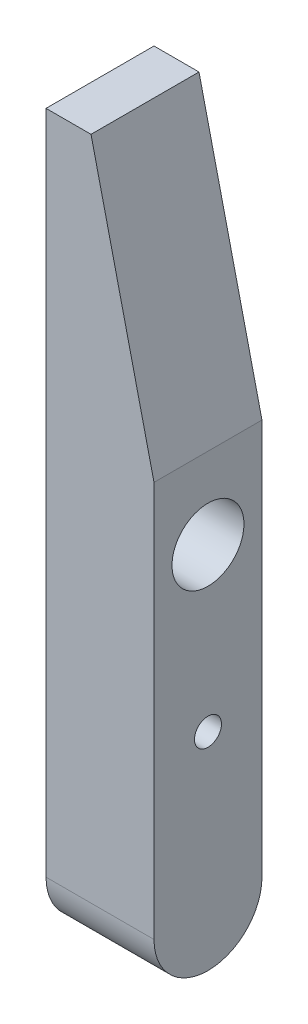
ISO-10303-21;
HEADER;
FILE_DESCRIPTION(('STEP AP214'),'2;1');
FILE_NAME('part.step','',(''),(''),'','','');
FILE_SCHEMA(('AUTOMOTIVE_DESIGN { 1 0 10303 214 1 1 1 1 }'));
ENDSEC;
DATA;
#1=APPLICATION_CONTEXT('core data for automotive mechanical design processes');
#2=APPLICATION_PROTOCOL_DEFINITION('international standard','automotive_design',2000,#1);
#3=PRODUCT_CONTEXT('',#1,'mechanical');
#4=PRODUCT('Part','Part','',(#3));
#5=PRODUCT_RELATED_PRODUCT_CATEGORY('part','',(#4));
#6=PRODUCT_DEFINITION_FORMATION('','',#4);
#7=PRODUCT_DEFINITION_CONTEXT('part definition',#1,'design');
#8=PRODUCT_DEFINITION('design','',#6,#7);
#9=PRODUCT_DEFINITION_SHAPE('','',#8);
#10=(LENGTH_UNIT() NAMED_UNIT(*) SI_UNIT(.MILLI.,.METRE.));
#11=(NAMED_UNIT(*) PLANE_ANGLE_UNIT() SI_UNIT($,.RADIAN.));
#12=(NAMED_UNIT(*) SI_UNIT($,.STERADIAN.) SOLID_ANGLE_UNIT());
#13=UNCERTAINTY_MEASURE_WITH_UNIT(LENGTH_MEASURE(1.E-05),#10,'distance_accuracy_value','');
#14=(GEOMETRIC_REPRESENTATION_CONTEXT(3) GLOBAL_UNCERTAINTY_ASSIGNED_CONTEXT((#13)) GLOBAL_UNIT_ASSIGNED_CONTEXT((#10,
#11,#12)) REPRESENTATION_CONTEXT('',''));
#15=CARTESIAN_POINT('',(0.,0.,0.));
#16=DIRECTION('',(0.,0.,1.));
#17=DIRECTION('',(1.,0.,0.));
#18=AXIS2_PLACEMENT_3D('',#15,#16,#17);
#19=CARTESIAN_POINT('',(0.,-74.,6.));
#20=DIRECTION('',(1.,0.,0.));
#21=DIRECTION('',(0.,0.,-1.));
#22=AXIS2_PLACEMENT_3D('',#19,#20,#21);
#23=PLANE('',#22);
#24=CARTESIAN_POINT('',(0.,-39.,0.));
#25=DIRECTION('',(1.,0.,0.));
#26=DIRECTION('',(0.,0.,-1.));
#27=AXIS2_PLACEMENT_3D('',#24,#25,#26);
#28=CIRCLE('',#27,4.);
#29=CARTESIAN_POINT('',(0.,-39.,-4.));
#30=VERTEX_POINT('',#29);
#31=EDGE_CURVE('E141',#30,#30,#28,.T.);
#32=ORIENTED_EDGE('',*,*,#31,.T.);
#33=EDGE_LOOP('',(#32));
#34=FACE_BOUND('',#33,.T.);
#35=CARTESIAN_POINT('',(0.,-74.,0.));
#36=DIRECTION('',(-1.,0.,0.));
#37=DIRECTION('',(0.,0.,1.));
#38=AXIS2_PLACEMENT_3D('',#35,#36,#37);
#39=CIRCLE('',#38,2.4);
#40=CARTESIAN_POINT('',(0.,-74.,2.4));
#41=VERTEX_POINT('',#40);
#42=EDGE_CURVE('E138',#41,#41,#39,.T.);
#43=ORIENTED_EDGE('',*,*,#42,.F.);
#44=EDGE_LOOP('',(#43));
#45=FACE_BOUND('',#44,.T.);
#46=DIRECTION('',(0.,-1.,0.));
#47=VECTOR('',#46,1.);
#48=CARTESIAN_POINT('',(0.,-74.,-6.));
#49=LINE('',#48,#47);
#50=CARTESIAN_POINT('',(0.,0.,-6.));
#51=VERTEX_POINT('',#50);
#52=CARTESIAN_POINT('',(0.,-74.,-6.));
#53=VERTEX_POINT('',#52);
#54=EDGE_CURVE('E112',#51,#53,#49,.T.);
#55=ORIENTED_EDGE('',*,*,#54,.T.);
#56=CARTESIAN_POINT('',(0.,-74.,0.));
#57=DIRECTION('',(-1.,0.,0.));
#58=DIRECTION('',(0.,0.,1.));
#59=AXIS2_PLACEMENT_3D('',#56,#57,#58);
#60=CIRCLE('',#59,6.);
#61=CARTESIAN_POINT('',(0.,-74.,6.));
#62=VERTEX_POINT('',#61);
#63=EDGE_CURVE('E132',#53,#62,#60,.T.);
#64=ORIENTED_EDGE('',*,*,#63,.T.);
#65=DIRECTION('',(0.,-1.,0.));
#66=VECTOR('',#65,1.);
#67=CARTESIAN_POINT('',(0.,-74.,6.));
#68=LINE('',#67,#66);
#69=CARTESIAN_POINT('',(0.,0.,6.));
#70=VERTEX_POINT('',#69);
#71=EDGE_CURVE('E89',#70,#62,#68,.T.);
#72=ORIENTED_EDGE('',*,*,#71,.F.);
#73=DIRECTION('',(0.,0.,-1.));
#74=VECTOR('',#73,1.);
#75=CARTESIAN_POINT('',(0.,0.,6.));
#76=LINE('',#75,#74);
#77=EDGE_CURVE('E109',#70,#51,#76,.T.);
#78=ORIENTED_EDGE('',*,*,#77,.T.);
#79=EDGE_LOOP('',(#55,#64,#72,#78));
#80=FACE_BOUND('',#79,.T.);
#81=ADVANCED_FACE('F43',(#34,#45,#80),#23,.F.);
#82=CARTESIAN_POINT('',(12.,-30.,6.));
#83=DIRECTION('',(-1.,0.,0.));
#84=DIRECTION('',(0.,-1.,0.));
#85=AXIS2_PLACEMENT_3D('',#82,#83,#84);
#86=PLANE('',#85);
#87=CARTESIAN_POINT('',(12.,-57.,0.));
#88=DIRECTION('',(1.,0.,0.));
#89=DIRECTION('',(0.,0.,-1.));
#90=AXIS2_PLACEMENT_3D('',#87,#88,#89);
#91=CIRCLE('',#90,1.5);
#92=CARTESIAN_POINT('',(12.,-57.,-1.5));
#93=VERTEX_POINT('',#92);
#94=EDGE_CURVE('E154',#93,#93,#91,.T.);
#95=ORIENTED_EDGE('',*,*,#94,.F.);
#96=EDGE_LOOP('',(#95));
#97=FACE_BOUND('',#96,.T.);
#98=CARTESIAN_POINT('',(12.,-39.,0.));
#99=DIRECTION('',(1.,0.,0.));
#100=DIRECTION('',(0.,0.,-1.));
#101=AXIS2_PLACEMENT_3D('',#98,#99,#100);
#102=CIRCLE('',#101,4.);
#103=CARTESIAN_POINT('',(12.,-39.,-4.));
#104=VERTEX_POINT('',#103);
#105=EDGE_CURVE('E150',#104,#104,#102,.T.);
#106=ORIENTED_EDGE('',*,*,#105,.F.);
#107=EDGE_LOOP('',(#106));
#108=FACE_BOUND('',#107,.T.);
#109=DIRECTION('',(0.,1.,0.));
#110=VECTOR('',#109,1.);
#111=CARTESIAN_POINT('',(12.,-30.,6.));
#112=LINE('',#111,#110);
#113=CARTESIAN_POINT('',(12.,-74.,6.));
#114=VERTEX_POINT('',#113);
#115=CARTESIAN_POINT('',(12.,-30.,6.));
#116=VERTEX_POINT('',#115);
#117=EDGE_CURVE('E94',#114,#116,#112,.T.);
#118=ORIENTED_EDGE('',*,*,#117,.F.);
#119=CARTESIAN_POINT('',(12.,-74.,0.));
#120=DIRECTION('',(-1.,0.,0.));
#121=DIRECTION('',(0.,-1.,0.));
#122=AXIS2_PLACEMENT_3D('',#119,#120,#121);
#123=CIRCLE('',#122,6.);
#124=CARTESIAN_POINT('',(12.,-74.,-6.));
#125=VERTEX_POINT('',#124);
#126=EDGE_CURVE('E117',#114,#125,#123,.F.);
#127=ORIENTED_EDGE('',*,*,#126,.T.);
#128=DIRECTION('',(0.,1.,0.));
#129=VECTOR('',#128,1.);
#130=CARTESIAN_POINT('',(12.,-30.,-6.));
#131=LINE('',#130,#129);
#132=CARTESIAN_POINT('',(12.,-30.,-6.));
#133=VERTEX_POINT('',#132);
#134=EDGE_CURVE('E110',#125,#133,#131,.T.);
#135=ORIENTED_EDGE('',*,*,#134,.T.);
#136=DIRECTION('',(0.,0.,-1.));
#137=VECTOR('',#136,1.);
#138=CARTESIAN_POINT('',(12.,-30.,6.));
#139=LINE('',#138,#137);
#140=EDGE_CURVE('E11',#116,#133,#139,.T.);
#141=ORIENTED_EDGE('',*,*,#140,.F.);
#142=EDGE_LOOP('',(#118,#127,#135,#141));
#143=FACE_BOUND('',#142,.T.);
#144=ADVANCED_FACE('F102',(#97,#108,#143),#86,.F.);
#145=CARTESIAN_POINT('',(5.,0.,6.));
#146=DIRECTION('',(-0.973841209741793,-0.227229615606418,0.));
#147=DIRECTION('',(0.227229615606418,-0.973841209741793,0.));
#148=AXIS2_PLACEMENT_3D('',#145,#146,#147);
#149=PLANE('',#148);
#150=DIRECTION('',(-0.227229615606418,0.973841209741793,0.));
#151=VECTOR('',#150,1.);
#152=CARTESIAN_POINT('',(5.,0.,-6.));
#153=LINE('',#152,#151);
#154=CARTESIAN_POINT('',(5.,0.,-6.));
#155=VERTEX_POINT('',#154);
#156=EDGE_CURVE('E77',#133,#155,#153,.T.);
#157=ORIENTED_EDGE('',*,*,#156,.T.);
#158=DIRECTION('',(0.,0.,-1.));
#159=VECTOR('',#158,1.);
#160=CARTESIAN_POINT('',(5.,0.,6.));
#161=LINE('',#160,#159);
#162=CARTESIAN_POINT('',(5.,0.,6.));
#163=VERTEX_POINT('',#162);
#164=EDGE_CURVE('E51',#163,#155,#161,.T.);
#165=ORIENTED_EDGE('',*,*,#164,.F.);
#166=DIRECTION('',(-0.227229615606418,0.973841209741793,0.));
#167=VECTOR('',#166,1.);
#168=CARTESIAN_POINT('',(5.,0.,6.));
#169=LINE('',#168,#167);
#170=EDGE_CURVE('E100',#116,#163,#169,.T.);
#171=ORIENTED_EDGE('',*,*,#170,.F.);
#172=ORIENTED_EDGE('',*,*,#140,.T.);
#173=EDGE_LOOP('',(#157,#165,#171,#172));
#174=FACE_BOUND('',#173,.T.);
#175=ADVANCED_FACE('F108',(#174),#149,.F.);
#176=CARTESIAN_POINT('',(0.,0.,6.));
#177=DIRECTION('',(0.,-1.,0.));
#178=DIRECTION('',(0.,0.,-1.));
#179=AXIS2_PLACEMENT_3D('',#176,#177,#178);
#180=PLANE('',#179);
#181=DIRECTION('',(-1.,0.,0.));
#182=VECTOR('',#181,1.);
#183=CARTESIAN_POINT('',(0.,0.,-6.));
#184=LINE('',#183,#182);
#185=EDGE_CURVE('E85',#155,#51,#184,.T.);
#186=ORIENTED_EDGE('',*,*,#185,.T.);
#187=ORIENTED_EDGE('',*,*,#77,.F.);
#188=DIRECTION('',(-1.,0.,0.));
#189=VECTOR('',#188,1.);
#190=CARTESIAN_POINT('',(0.,0.,6.));
#191=LINE('',#190,#189);
#192=EDGE_CURVE('E56',#163,#70,#191,.T.);
#193=ORIENTED_EDGE('',*,*,#192,.F.);
#194=ORIENTED_EDGE('',*,*,#164,.T.);
#195=EDGE_LOOP('',(#186,#187,#193,#194));
#196=FACE_BOUND('',#195,.T.);
#197=ADVANCED_FACE('F121',(#196),#180,.F.);
#198=CARTESIAN_POINT('',(0.,0.,6.));
#199=DIRECTION('',(0.,0.,-1.));
#200=DIRECTION('',(-1.,0.,0.));
#201=AXIS2_PLACEMENT_3D('',#198,#199,#200);
#202=PLANE('',#201);
#203=ORIENTED_EDGE('',*,*,#71,.T.);
#204=DIRECTION('',(1.,0.,0.));
#205=VECTOR('',#204,1.);
#206=CARTESIAN_POINT('',(12.,-74.,6.));
#207=LINE('',#206,#205);
#208=EDGE_CURVE('E99',#62,#114,#207,.T.);
#209=ORIENTED_EDGE('',*,*,#208,.T.);
#210=ORIENTED_EDGE('',*,*,#117,.T.);
#211=ORIENTED_EDGE('',*,*,#170,.T.);
#212=ORIENTED_EDGE('',*,*,#192,.T.);
#213=EDGE_LOOP('',(#203,#209,#210,#211,#212));
#214=FACE_BOUND('',#213,.T.);
#215=ADVANCED_FACE('F97',(#214),#202,.F.);
#216=CARTESIAN_POINT('',(0.,0.,-6.));
#217=DIRECTION('',(0.,0.,-1.));
#218=DIRECTION('',(-1.,0.,0.));
#219=AXIS2_PLACEMENT_3D('',#216,#217,#218);
#220=PLANE('',#219);
#221=ORIENTED_EDGE('',*,*,#54,.F.);
#222=ORIENTED_EDGE('',*,*,#185,.F.);
#223=ORIENTED_EDGE('',*,*,#156,.F.);
#224=ORIENTED_EDGE('',*,*,#134,.F.);
#225=DIRECTION('',(1.,0.,0.));
#226=VECTOR('',#225,1.);
#227=CARTESIAN_POINT('',(12.,-74.,-6.));
#228=LINE('',#227,#226);
#229=EDGE_CURVE('E120',#53,#125,#228,.T.);
#230=ORIENTED_EDGE('',*,*,#229,.F.);
#231=EDGE_LOOP('',(#221,#222,#223,#224,#230));
#232=FACE_BOUND('',#231,.T.);
#233=ADVANCED_FACE('F130',(#232),#220,.T.);
#234=CARTESIAN_POINT('',(28.9705627484772,-74.,0.));
#235=DIRECTION('',(-1.,0.,0.));
#236=DIRECTION('',(0.,0.,1.));
#237=AXIS2_PLACEMENT_3D('',#234,#235,#236);
#238=CYLINDRICAL_SURFACE('',#237,6.);
#239=ORIENTED_EDGE('',*,*,#126,.F.);
#240=ORIENTED_EDGE('',*,*,#208,.F.);
#241=ORIENTED_EDGE('',*,*,#63,.F.);
#242=ORIENTED_EDGE('',*,*,#229,.T.);
#243=EDGE_LOOP('',(#239,#240,#241,#242));
#244=FACE_BOUND('',#243,.T.);
#245=ADVANCED_FACE('F134',(#244),#238,.T.);
#246=CARTESIAN_POINT('',(6.,-74.,0.));
#247=DIRECTION('',(-1.,0.,0.));
#248=DIRECTION('',(0.,0.,1.));
#249=AXIS2_PLACEMENT_3D('',#246,#247,#248);
#250=CYLINDRICAL_SURFACE('',#249,2.4);
#251=CARTESIAN_POINT('',(6.,-74.,0.));
#252=DIRECTION('',(-1.,0.,0.));
#253=DIRECTION('',(0.,0.,1.));
#254=AXIS2_PLACEMENT_3D('',#251,#252,#253);
#255=CIRCLE('',#254,2.4);
#256=CARTESIAN_POINT('',(6.,-74.,2.4));
#257=VERTEX_POINT('',#256);
#258=EDGE_CURVE('E131',#257,#257,#255,.T.);
#259=ORIENTED_EDGE('',*,*,#258,.F.);
#260=EDGE_LOOP('',(#259));
#261=FACE_BOUND('',#260,.T.);
#262=ORIENTED_EDGE('',*,*,#42,.T.);
#263=EDGE_LOOP('',(#262));
#264=FACE_BOUND('',#263,.T.);
#265=ADVANCED_FACE('F174',(#261,#264),#250,.F.);
#266=CARTESIAN_POINT('',(6.,-74.,0.));
#267=DIRECTION('',(-1.,0.,0.));
#268=DIRECTION('',(0.,0.,1.));
#269=AXIS2_PLACEMENT_3D('',#266,#267,#268);
#270=PLANE('',#269);
#271=ORIENTED_EDGE('',*,*,#258,.T.);
#272=EDGE_LOOP('',(#271));
#273=FACE_BOUND('',#272,.T.);
#274=ADVANCED_FACE('F170',(#273),#270,.T.);
#275=CARTESIAN_POINT('',(12.,-39.,0.));
#276=DIRECTION('',(1.,0.,0.));
#277=DIRECTION('',(0.,0.,-1.));
#278=AXIS2_PLACEMENT_3D('',#275,#276,#277);
#279=CYLINDRICAL_SURFACE('',#278,4.);
#280=ORIENTED_EDGE('',*,*,#105,.T.);
#281=EDGE_LOOP('',(#280));
#282=FACE_BOUND('',#281,.T.);
#283=ORIENTED_EDGE('',*,*,#31,.F.);
#284=EDGE_LOOP('',(#283));
#285=FACE_BOUND('',#284,.T.);
#286=ADVANCED_FACE('F161',(#282,#285),#279,.F.);
#287=CARTESIAN_POINT('',(4.,-57.,0.));
#288=DIRECTION('',(1.,0.,0.));
#289=DIRECTION('',(0.,0.,-1.));
#290=AXIS2_PLACEMENT_3D('',#287,#288,#289);
#291=CONICAL_SURFACE('',#290,1.5,1.02974425867665);
#292=CARTESIAN_POINT('',(3.09870907145866,-57.,0.));
#293=VERTEX_POINT('',#292);
#294=VERTEX_LOOP('',#293);
#295=FACE_BOUND('',#294,.T.);
#296=CARTESIAN_POINT('',(4.,-57.,0.));
#297=DIRECTION('',(1.,0.,0.));
#298=DIRECTION('',(0.,0.,-1.));
#299=AXIS2_PLACEMENT_3D('',#296,#297,#298);
#300=CIRCLE('',#299,1.5);
#301=CARTESIAN_POINT('',(4.,-57.,-1.5));
#302=VERTEX_POINT('',#301);
#303=EDGE_CURVE('E148',#302,#302,#300,.T.);
#304=ORIENTED_EDGE('',*,*,#303,.T.);
#305=EDGE_LOOP('',(#304));
#306=FACE_BOUND('',#305,.T.);
#307=ADVANCED_FACE('F168',(#295,#306),#291,.F.);
#308=CARTESIAN_POINT('',(12.,-57.,0.));
#309=DIRECTION('',(1.,0.,0.));
#310=DIRECTION('',(0.,0.,-1.));
#311=AXIS2_PLACEMENT_3D('',#308,#309,#310);
#312=CYLINDRICAL_SURFACE('',#311,1.5);
#313=ORIENTED_EDGE('',*,*,#303,.F.);
#314=EDGE_LOOP('',(#313));
#315=FACE_BOUND('',#314,.T.);
#316=ORIENTED_EDGE('',*,*,#94,.T.);
#317=EDGE_LOOP('',(#316));
#318=FACE_BOUND('',#317,.T.);
#319=ADVANCED_FACE('F160',(#315,#318),#312,.F.);
#320=CLOSED_SHELL('',(#81,#144,#175,#197,#215,#233,#245,#265,#274,#286,#307,#319));
#321=MANIFOLD_SOLID_BREP('B2',#320);
#322=ADVANCED_BREP_SHAPE_REPRESENTATION('',(#18,#321),#14);
#323=SHAPE_DEFINITION_REPRESENTATION(#9,#322);
ENDSEC;
END-ISO-10303-21;
